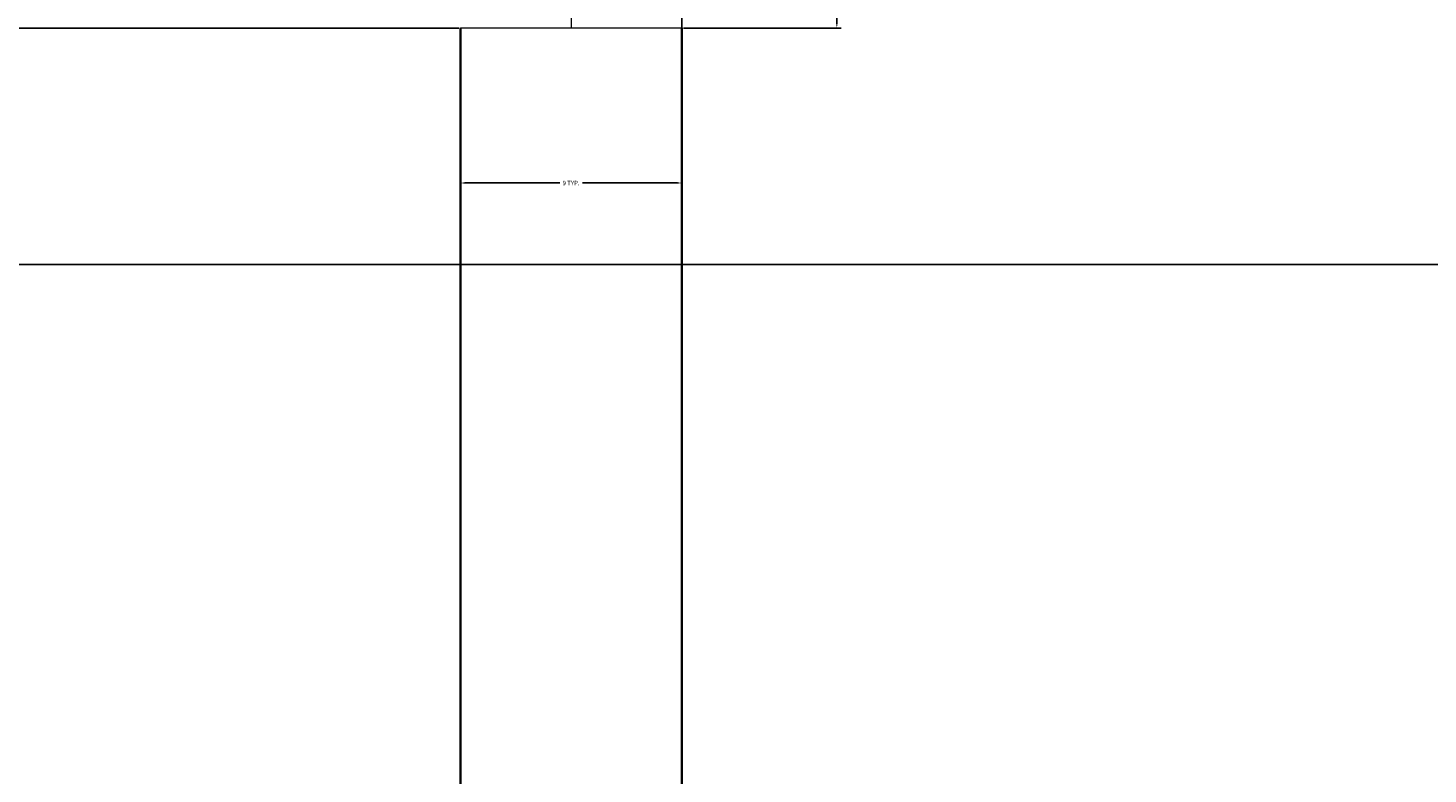
# Model space of a CAD drawing. Units: feet. Extents: x 1654 to 2985, y 1348 to 2230.
# Tile 33 of 53: x 2044 to 2100, y 1781 to 1811. Entities that reach past the tile are written whole.
import ezdxf

# ---------------------------------------------------------------- set-up
doc = ezdxf.new("R2010")
doc.units = ezdxf.units.FT
for name, color, linetype, lineweight in [('A-ANNO-DIMS', 2, 'Continuous', 18), ('A-WALL', 7, 'Continuous', 35), ('A-WALL-OPEN', 4, 'Continuous', 18)]:
    doc.layers.add(name, color=color, linetype=linetype, lineweight=lineweight)
doc.styles.get("Standard").update_dxf_attribs({"font": 'arial.ttf'})
doc.dimstyles.get("Standard").update_dxf_attribs({"dimtxt": 0.18, "dimasz": 0.18, "dimexe": 0.18, "dimexo": 0.0625, "dimgap": 0.09, "dimtad": 0, "dimtih": 1, "dimtoh": 1, "dimdec": 4, "dimzin": 0, "dimdsep": 46, "dimtxsty": 'Standard', "dimcen": 0.09, "dimadec": 0, "dimazin": 0, "dimtfac": 1, "dimtdec": 4, "dimtofl": 0, "dimtmove": 0, "dimatfit": 3, "dimfxl": 1, "dimtolj": 1, "dimtzin": 0, "dimarcsym": 0})

# ---------------------------------------------------------------- blocks, each defined once
blk = doc.blocks.new('OPENING-LIVING-ARCH')
for p, q in [((0, 42), (9, 42)), ((4.5, 42), (4.5, 0)), ((9, 0), (0, 0))]:
    blk.add_line(p, q)
blk = doc.blocks.new('*D70')
at = {"layer": 'A-ANNO-DIMS', "color": 0, "lineweight": -2, "transparency": 16777216}
for p, q in [((2070.155, 1853.081), (2076.572, 1853.081)), ((2076.392, 1852.901), (2076.392, 1832.265)), ((2076.392, 1811.261), (2076.392, 1831.898)), ((2070.155, 1811.081), (2076.572, 1811.081))]:
    blk.add_line(p, q, dxfattribs=at)
at = {"layer": 'A-ANNO-DIMS', "color": 0, "transparency": 16777216}
for points in [[(2076.362, 1852.901), (2076.422, 1852.901), (2076.392, 1853.081)], [(2076.362, 1811.261), (2076.422, 1811.261), (2076.392, 1811.081)]]:
    blk.add_solid(points, dxfattribs=at)
at = {"layer": 'Defpoints', "color": 0, "transparency": 16777216}
for p in [(2070.092, 1853.081), (2076.392, 1853.081), (2070.092, 1811.081)]:
    blk.add_point(p, dxfattribs=at)
at = {"layer": 'A-ANNO-DIMS', "color": 0, "transparency": 16777216, "insert": (2076.392, 1832.081), "char_height": 0.18, "attachment_point": 5}
blk.add_mtext('\\A1;ARCH 42 TYP.', dxfattribs=at)
blk = doc.blocks.new('*D71')
at = {"layer": 'A-ANNO-DIMS', "color": 0, "lineweight": -2, "transparency": 16777216}
for p, q in [((2061.092, 1811.019), (2061.092, 1804.601)), ((2070.092, 1811.019), (2070.092, 1804.601)), ((2061.272, 1804.781), (2065.134, 1804.781)), ((2069.912, 1804.781), (2066.051, 1804.781))]:
    blk.add_line(p, q, dxfattribs=at)
at = {"layer": 'A-ANNO-DIMS', "color": 0, "transparency": 16777216}
for points in [[(2061.272, 1804.811), (2061.272, 1804.751), (2061.092, 1804.781)], [(2069.912, 1804.811), (2069.912, 1804.751), (2070.092, 1804.781)]]:
    blk.add_solid(points, dxfattribs=at)
at = {"layer": 'Defpoints', "color": 0, "transparency": 16777216}
for p in [(2061.092, 1811.081), (2070.092, 1811.081), (2070.092, 1804.781)]:
    blk.add_point(p, dxfattribs=at)
at = {"layer": 'A-ANNO-DIMS', "color": 0, "transparency": 16777216, "insert": (2065.592, 1804.781), "char_height": 0.18, "attachment_point": 5}
blk.add_mtext('\\A1;9 TYP.', dxfattribs=at)
blk = doc.blocks.new('*D80')
at = {"layer": 'A-ANNO-DIMS', "color": 0, "lineweight": -2, "transparency": 16777216}
for p, q in [((2070.092, 2039.192), (2070.092, 1534.075)), ((2202.092, 2039.192), (2202.092, 1534.075)), ((2070.272, 1534.255), (2135.813, 1534.255)), ((2201.912, 1534.255), (2136.372, 1534.255))]:
    blk.add_line(p, q, dxfattribs=at)
at = {"layer": 'A-ANNO-DIMS', "color": 0, "transparency": 16777216}
for points in [[(2070.272, 1534.285), (2070.272, 1534.225), (2070.092, 1534.255)], [(2201.912, 1534.285), (2201.912, 1534.225), (2202.092, 1534.255)]]:
    blk.add_solid(points, dxfattribs=at)
at = {"layer": 'Defpoints', "color": 0, "transparency": 16777216}
for p in [(2070.092, 2039.255), (2202.092, 2039.255), (2202.092, 1534.255)]:
    blk.add_point(p, dxfattribs=at)
at = {"layer": 'A-ANNO-DIMS', "color": 0, "transparency": 16777216, "insert": (2136.092, 1534.255), "char_height": 0.18, "attachment_point": 5}
blk.add_mtext('\\A1;132', dxfattribs=at)
blk = doc.blocks.new('*D91')
at = {"layer": 'A-ANNO-DIMS', "color": 0, "lineweight": -2, "transparency": 16777216}
for p, q in [((1852.155, 1801.468), (2242.272, 1801.468)), ((2242.092, 1801.288), (2242.092, 1776.544)), ((2242.092, 1751.435), (2242.092, 1776.18)), ((1852.155, 1751.255), (2242.272, 1751.255))]:
    blk.add_line(p, q, dxfattribs=at)
at = {"layer": 'A-ANNO-DIMS', "color": 0, "transparency": 16777216}
for points in [[(2242.062, 1801.288), (2242.122, 1801.288), (2242.092, 1801.468)], [(2242.062, 1751.435), (2242.122, 1751.435), (2242.092, 1751.255)]]:
    blk.add_solid(points, dxfattribs=at)
at = {"layer": 'Defpoints', "color": 0, "transparency": 16777216}
for p in [(1852.092, 1801.468), (2242.092, 1801.468), (1852.092, 1751.255)]:
    blk.add_point(p, dxfattribs=at)
at = {"layer": 'A-ANNO-DIMS', "color": 0, "transparency": 16777216, "insert": (2242.092, 1776.362), "char_height": 0.18, "attachment_point": 5}
blk.add_mtext('\\A1;50.21', dxfattribs=at)
blk = doc.blocks.new('*D98')
at = {"layer": 'A-ANNO-DIMS', "color": 0, "lineweight": -2, "transparency": 16777216}
for p, q in [((2061.03, 1811.081), (1811.912, 1811.081)), ((1812.092, 1810.901), (1812.092, 1781.35)), ((1812.092, 1751.435), (1812.092, 1780.986)), ((2061.03, 1751.255), (1811.912, 1751.255))]:
    blk.add_line(p, q, dxfattribs=at)
at = {"layer": 'A-ANNO-DIMS', "color": 0, "transparency": 16777216}
for points in [[(1812.062, 1810.901), (1812.122, 1810.901), (1812.092, 1811.081)], [(1812.062, 1751.435), (1812.122, 1751.435), (1812.092, 1751.255)]]:
    blk.add_solid(points, dxfattribs=at)
at = {"layer": 'Defpoints', "color": 0, "transparency": 16777216}
for p in [(1812.092, 1811.081), (2061.092, 1811.081), (2061.092, 1751.255)]:
    blk.add_point(p, dxfattribs=at)
at = {"layer": 'A-ANNO-DIMS', "color": 0, "transparency": 16777216, "insert": (1812.092, 1781.168), "char_height": 0.18, "attachment_point": 5}
blk.add_mtext('\\A1;59.83', dxfattribs=at)

msp = doc.modelspace()

# ---------------------------------------------------------------- linework, layer by layer
at = {"layer": 'A-WALL'}
for p, q in [((2061.0924, 1751.2549), (2061.0924, 1811.0815)), ((2070.0924, 1751.2549), (2070.0924, 1811.0815))]:
    msp.add_line(p, q, dxfattribs=at)

# ---------------------------------------------------------------- block references
at = {"layer": 'A-WALL-OPEN'}
msp.add_blockref('OPENING-LIVING-ARCH', (2061.092, 1811.081), dxfattribs=at)

# ---------------------------------------------------------------- dimensions: what is measured, and where the dimension line sits
at = {"layer": 'A-ANNO-DIMS'}
dim = msp.add_linear_dim(base=(2202.0924, 1534.2549), p1=(2070.0924, 2039.2549), p2=(2202.0924, 2039.2549), dimstyle='Standard', override={"dimdec": 0, "dimlfac": 1, "dimrnd": 0, "dimzin": 0, "dimdsep": 46, "dimlunit": 2}, dxfattribs=at)
dim.commit()
dim.dimension.update_dxf_attribs({"geometry": '*D80', "text_midpoint": (2136.0924, 1534.2549)})
dim = msp.add_linear_dim(base=(2076.3924, 1853.0815), p1=(2070.0924, 1811.0815), p2=(2070.0924, 1853.0815), angle=90, text='ARCH <> TYP.', dimstyle='Standard', override={"dimdec": 0, "dimlfac": 1, "dimrnd": 0, "dimzin": 0, "dimdsep": 46, "dimlunit": 2}, dxfattribs=at)
dim.commit()
dim.dimension.update_dxf_attribs({"geometry": '*D70', "text_midpoint": (2076.3924, 1832.0815)})
for base, p1, p2, picture, middle in [((1812.0924, 1811.0815), (2061.0924, 1751.2549), (2061.0924, 1811.0815), '*D98', (1812.0924, 1781.1682)), ((2242.0924, 1801.4683), (1852.0924, 1751.2549), (1852.0924, 1801.4683), '*D91', (2242.0924, 1776.3616))]:
    dim = msp.add_linear_dim(base=base, p1=p1, p2=p2, angle=90, dimstyle='Standard', override={"dimdec": 2, "dimlfac": 1, "dimrnd": 0, "dimzin": 0, "dimdsep": 46, "dimlunit": 2}, dxfattribs=at)
    dim.commit()
    dim.dimension.update_dxf_attribs({"geometry": picture, "text_midpoint": middle})
dim = msp.add_linear_dim(base=(2070.0924, 1804.7815), p1=(2061.0924, 1811.0815), p2=(2070.0924, 1811.0815), text='<> TYP.', dimstyle='Standard', override={"dimdec": 0, "dimlfac": 1, "dimrnd": 0, "dimzin": 0, "dimdsep": 46, "dimlunit": 2}, dxfattribs=at)
dim.commit()
dim.dimension.update_dxf_attribs({"geometry": '*D71', "text_midpoint": (2065.5924, 1804.7815)})

doc.saveas('drawing.dxf')
